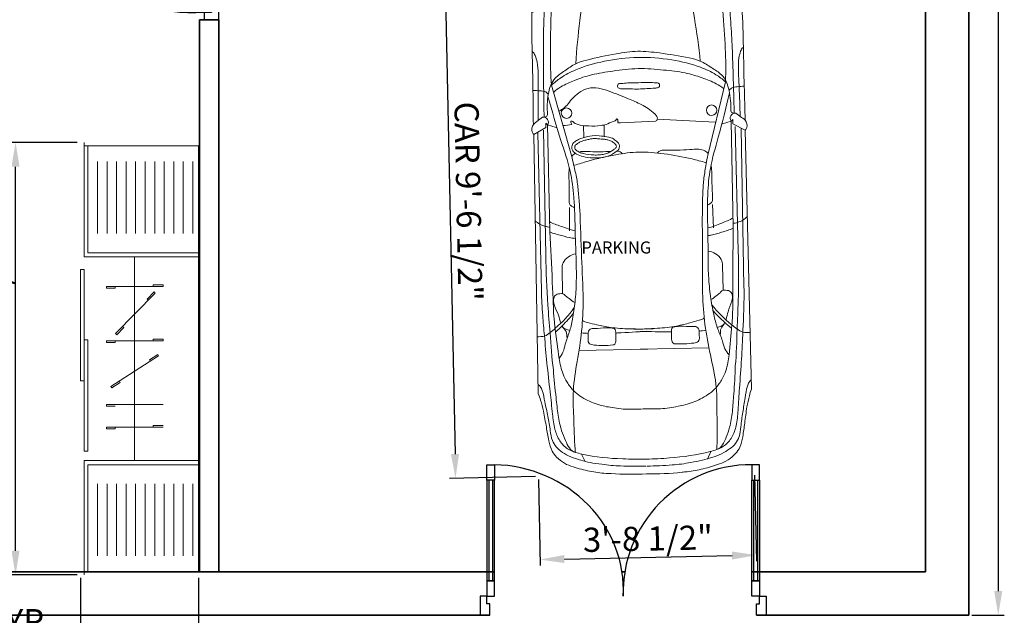
# Model space of a CAD drawing. Units: inches. Extents: x -24887 to 3061, y 1794 to 4919553.
# Tile 10 of 14: x 2858 to 3061, y 1957 to 2080. Entities that reach past the tile are written whole.
import ezdxf

# ---------------------------------------------------------------- set-up
doc = ezdxf.new("R2010")
doc.units = ezdxf.units.IN
for name, color, linetype, lineweight in [('A-ANNO-DIMS', 2, 'Continuous', 18), ('A-AREA-IDEN', 7, 'Continuous', 18), ('A-FLOR-PRKG', 8, 'Continuous', 13), ('A-FURN', 8, 'Continuous', 18), ('door', 4, 'Continuous', 25), ('wall', 7, 'Continuous', 35)]:
    doc.layers.add(name, color=color, linetype=linetype, lineweight=lineweight)
doc.styles.get("Standard").update_dxf_attribs({"font": 'arial.ttf'})
doc.dimstyles.new('ISO-25', dxfattribs={"dimtxt": 5, "dimasz": 5, "dimexe": 1.25, "dimexo": 0.625, "dimtad": 1, "dimdec": 1, "dimlunit": 3, "dimtxsty": 'Standard', "dimcen": 2.5, "dimadec": 0, "dimazin": 0, "dimtfac": 1, "dimtdec": 1, "dimtmove": 0, "dimatfit": 3, "dimfxl": 1, "dimarcsym": 0})

# ---------------------------------------------------------------- blocks, each defined once
blk = doc.blocks.new('A$C34930FF8')
at = {"ltscale": 0.05}
for p, q in [((0, 2252.4), (0, 16.8)), ((600, 2252.4), (0, 2252.4)), ((185.4, 1513), (185.4, 1521.5)), ((237.7, 1513), (237.7, 1521.5)), ((436.7, 1513), (436.7, 1504.4)), ((482.5, 1513), (482.5, 1504.4)), ((227.1, 1479.2), (233.2, 1485.2)), ((263.6, 1441.7), (269.7, 1447.7)), ((398.2, 1303.6), (392.1, 1297.6)), ((434.8, 1266.1), (428.7, 1260.1)), ((185.4, 1229.1), (185.4, 1237.7)), ((237.7, 1229.1), (237.7, 1237.7)), ((436.7, 1228.2), (436.7, 1219.7)), ((482.5, 1228.2), (482.5, 1219.7)), ((209.5, 1150.1), (214.1, 1157.3)), ((253.5, 1121.8), (258.1, 1129)), ((415.3, 1017.6), (410.6, 1010.5)), ((459.3, 989.3), (454.7, 982.1)), ((482.5, 894.9), (482.5, 886.3)), ((237.7, 775.3), (237.7, 783.9)), ((436.7, 775.3), (436.7, 766.8)), ((482.5, 775.3), (482.5, 766.8)), ((600, 16.8), (0, 16.8))]:
    blk.add_line(p, q, dxfattribs=at)
for p, q in [((580, 1690.9), (580, 2252.4)), ((600, 1669.3), (600, 2269.3)), ((30, 1790.9), (30, 2169.3)), ((80, 1790.9), (80, 2169.3)), ((130, 1790.9), (130, 2169.3)), ((180, 1790.9), (180, 2169.3)), ((230, 1790.9), (230, 2169.3)), ((280, 1790.9), (280, 2169.3)), ((330, 1790.9), (330, 2169.3)), ((380, 1790.9), (380, 2169.3)), ((430, 1790.9), (430, 2169.3)), ((480, 1790.9), (480, 2169.3)), ((530, 1790.9), (530, 2169.3)), ((580, 1690.9), (0, 1690.9)), ((600, 1669.3), (0, 1669.3)), ((335.4, 1666.1), (335.4, 603.1)), ((600, 1603.3), (620, 1603.3)), ((600, 1018.7), (600, 1603.3)), ((620, 1603.3), (620, 1018.7)), ((237.7, 1521.5), (185.4, 1521.5)), ((482.5, 1513), (185.4, 1513)), ((436.7, 1504.4), (482.5, 1504.4)), ((434.8, 1266.1), (227.4, 1478.9)), ((269.7, 1447.7), (233.2, 1485.2)), ((428.7, 1260.1), (392.1, 1297.6)), ((237.7, 1237.7), (185.4, 1237.7)), ((482.5, 1228.2), (185.4, 1228.2)), ((436.7, 1219.7), (482.5, 1219.7)), ((600, 1233.4), (580, 1233.4)), ((580, 1233.4), (580, 648.7)), ((600, 648.7), (600, 1233.4)), ((459.3, 989.3), (209.5, 1150.1)), ((258.1, 1129), (214.1, 1157.3)), ((454.7, 982.1), (410.6, 1010.5)), ((620, 1018.7), (600, 1018.7)), ((482.5, 894.9), (185.4, 894.9)), ((436.7, 886.3), (482.5, 886.3)), ((237.7, 783.9), (185.4, 783.9)), ((482.5, 775.3), (185.4, 775.3)), ((436.7, 766.8), (482.5, 766.8)), ((580, 648.7), (600, 648.7)), ((600, 600), (0, 600)), ((580, 578.3), (0, 578.3)), ((580, 578.3), (580, 16.8)), ((600, 600), (600, 0)), ((30, 478.3), (30, 100)), ((80, 478.3), (80, 100)), ((130, 478.3), (130, 100)), ((180, 478.3), (180, 100)), ((230, 478.3), (230, 100)), ((280, 478.3), (280, 100)), ((330, 478.3), (330, 100)), ((380, 478.3), (380, 100)), ((430, 478.3), (430, 100)), ((480, 478.3), (480, 100)), ((530, 478.3), (530, 100))]:
    blk.add_line(p, q)
blk = doc.blocks.new('A$C242571DA')
for p, q in [((1659.9, 1632), (1714.3, 1732.5)), ((1699.9, 1699.4), (2984.7, 1695.8)), ((1714.3, 1732.5), (3817.1, 1739.9)), ((1638.3, 1618.5), (1625.1, 1632)), ((1625.1, 1632), (1659.9, 1632)), ((1638.3, 1618.5), (2503.3, 1618.5)), ((1659.9, 1548.1), (1638.3, 1618.5)), ((1681.8, 1651.6), (2695.2, 1655.3)), ((2503.3, 1618.5), (2861.6, 1607.5)), ((1317.4, 1579.7), (1909.8, 1424.9)), ((3007.2, 1526.5), (2808.1, 1525.2)), ((1644, 1489.1), (1610.4, 1020.2)), ((2311.9, 1454.3), (2500.6, 1456.9)), ((3474.6, 1401.1), (3474.6, 843)), ((4315.2, 1398), (4377.3, 1370.5)), ((1626.1, 1006.5), (1632.8, 719.7)), ((3474.6, 345.6), (3474.6, 903.8)), ((1740.2, 584.9), (1649.3, 586.9)), ((1746.1, 420.6), (1649.3, 420.6)), ((1317.4, 167), (1909.8, 321.9)), ((4315.2, 348.7), (4377.3, 376.3)), ((2311.9, 292.5), (2500.6, 289.8)), ((1659.9, 198.7), (1638.3, 128.2)), ((3007.2, 220.3), (2808.1, 221.6)), ((1638.3, 128.2), (1625.1, 114.7)), ((1625.1, 114.7), (1659.9, 114.7)), ((1638.3, 128.2), (2503.3, 128.2)), ((1659.9, 114.7), (1714.3, 14.2)), ((1681.8, 95.1), (2695.2, 91.4)), ((2503.3, 128.2), (2861.6, 139.2)), ((1699.9, 47.3), (2984.7, 51)), ((1714.3, 14.2), (3817.1, 6.9))]:
    blk.add_line(p, q)
for centre in [(1546.4, 1462.5), (1546.4, 284.2)]:
    blk.add_ellipse(centre, major_axis=(0, 42.9), ratio=0.983266, start_param=4.712389, end_param=10.995574)
for points, knots in [([(0, 873.4), (0, 927.8), (15.6, 1088.6), (25.5, 1309.8), (120.7, 1476.4), (189.2, 1569), (273.5, 1623.1), (369.9, 1666.3), (483, 1694.7), (561.3, 1714.9), (604.6, 1715.7)], [0, 0, 0, 0, 0.16039, 0.479033, 0.632967, 0.722015, 0.817474, 0.927562, 1.03733, 1.167094, 1.167094, 1.167094, 1.167094]), ([(604.6, 1715.7), (545.5, 1714.5), (448.5, 1664.6), (320.8, 1610.6), (225.4, 1521.2), (147.3, 1390.5), (121.7, 1275.2), (113.6, 1208.7)], [0, 0, 0, 0, 0.1772572, 0.3124951, 0.4151678, 0.5597243, 0.7575412, 0.7575412, 0.7575412, 0.7575412]), ([(722.7, 1726.6), (720.8, 1714.9), (694.5, 1689.9), (643, 1671.8), (573.6, 1655.4), (508.5, 1647), (455.2, 1634.7), (428.7, 1627.3), (416.9, 1624.1)], [0, 0, 0, 0, 0.034703, 0.0959761, 0.1659336, 0.2471559, 0.2929944, 0.3295918, 0.3295918, 0.3295918, 0.3295918]), ([(604.6, 1715.7), (642.1, 1723.4), (788.5, 1729.2), (1039.3, 1732.2), (1344.5, 1729.9), (1542, 1733.1), (1633.8, 1733.7)], [0, 0, 0, 0, 0.114897, 0.437061, 0.754269, 1.029686, 1.029686, 1.029686, 1.029686]), ([(1043.6, 1729.2), (1048.6, 1717.9), (1080.9, 1704.2), (1138.6, 1687.6), (1237.7, 1685.6), (1394.7, 1691.3), (1521.7, 1692.4), (1601.5, 1692.7)], [0, 0, 0, 0, 0.0364992, 0.0923739, 0.1867837, 0.3273982, 0.5667068, 0.5667068, 0.5667068, 0.5667068]), ([(1356.8, 1732.2), (1357.1, 1712.8), (1360, 1678.8), (1363.9, 1630.5), (1383.3, 1613.5), (1391, 1607.2)], [0, 0, 0, 0, 1.462159, 2.651105, 3.386321, 3.386321, 3.386321, 3.386321]), ([(1714.3, 1732.5), (1707.7, 1737.6), (1683.3, 1753), (1628.7, 1741.2), (1605.6, 1691.5), (1561.7, 1652.4), (1594.1, 1610.3), (1627.9, 1608.3), (1638.3, 1618.5)], [0, 0, 0, 0, 0.024864, 0.0846267, 0.1362471, 0.1900683, 0.2245199, 0.2681841, 0.2681841, 0.2681841, 0.2681841]), ([(2414.7, 1735), (2424.9, 1723.3), (2447.2, 1698.8), (2461.2, 1657.6), (2468.1, 1629), (2468, 1616.1)], [1.808086, 1.808086, 1.808086, 1.808086, 2.918874, 4.131288, 5.10151, 5.10151, 5.10151, 5.10151]), ([(2984.7, 1695.8), (3051, 1695.6), (3172.1, 1691.3), (3367.4, 1677.6), (3575.2, 1664.3), (3788.2, 1643.6), (3968, 1628.1), (4103.8, 1616.8), (4203.6, 1578.1), (4271.8, 1519.5), (4300.6, 1452.1), (4341.7, 1305.3), (4361.8, 1111.2), (4367.5, 936.8), (4367.5, 873.4)], [0, 0, 0, 0, 0.198873, 0.363323, 0.587433, 0.823543, 1.004622, 1.129816, 1.230113, 1.320655, 1.388577, 1.443334, 1.771447, 1.958652, 1.958652, 1.958652, 1.958652]), ([(3356.5, 1739.4), (3354.9, 1719.2), (3360.8, 1678.2), (3324, 1631.5), (3255.4, 1544.3), (3187.1, 1476.2), (3125.2, 1432.2)], [0, 0, 0, 0, 0.0597371, 0.1139981, 0.1672498, 0.3938869, 0.3938869, 0.3938869, 0.3938869]), ([(3745.3, 1736.8), (3748.5, 1730.1), (3764.2, 1717.1), (3811.5, 1698.6), (3894.7, 1686.7), (4002.9, 1663.2), (4107.9, 1648.7), (4195.8, 1638.3), (4258.6, 1603.2), (4302.1, 1549.7), (4339.9, 1483.8), (4365.2, 1407.6), (4389.6, 1324.4), (4397.9, 1266.9), (4401.8, 1235.2)], [0, 0, 0, 0, 0.0219205, 0.0572122, 0.1522539, 0.2718866, 0.3894011, 0.4710097, 0.5346344, 0.5986698, 0.6733118, 0.758696, 0.8351341, 0.9293726, 0.9293726, 0.9293726, 0.9293726]), ([(3817.1, 1739.9), (3833.2, 1729.7), (3882.9, 1718.2), (3973.3, 1695.2), (4085.1, 1680.5), (4193.8, 1662.8), (4280.6, 1644.3), (4343.9, 1598.1), (4390, 1540.3), (4427.4, 1448.7), (4457.8, 1336.6), (4475.7, 1233.4), (4478.4, 1175.1), (4479.3, 1161.6)], [0, 0, 0, 0, 0.056668, 0.14946, 0.28161, 0.392935, 0.481686, 0.542967, 0.622845, 0.69797, 0.833643, 0.965665, 1.00577, 1.00577, 1.00577, 1.00577]), ([(310.7, 1637.3), (282.5, 1613.7), (230.1, 1569.9), (148.7, 1486.2), (84.8, 1361.3), (60, 1219), (32.6, 1054.3), (25.1, 944.9), (25.1, 873.4)], [0, 0, 0, 0, 0.1095129, 0.2035347, 0.3452507, 0.5161382, 0.6275464, 0.8383798, 0.8383798, 0.8383798, 0.8383798]), ([(426.8, 1656.7), (428.5, 1646.6), (426.9, 1625), (399.8, 1616.6), (368.1, 1593.9), (328, 1564.6), (271.6, 1523.9), (237, 1451.9), (196.2, 1376.7), (183.8, 1314.9), (170, 1279.6), (157.2, 1254.2), (133.3, 1244.4), (118.6, 1242.9)], [0, 0, 0, 0, 0.0304541, 0.0502818, 0.0786089, 0.1479133, 0.1986294, 0.2831705, 0.3780326, 0.4523267, 0.4667809, 0.4902599, 0.5347198, 0.5347198, 0.5347198, 0.5347198]), ([(323.7, 1557.5), (344.8, 1571.9), (400.4, 1585.1), (516, 1606.8), (680.3, 1625.8), (885.4, 1635.7), (1116.8, 1642.2), (1346.1, 1644.2), (1504.7, 1644.7), (1574, 1645.7)], [0, 0, 0, 0, 0.076148, 0.165903, 0.355672, 0.569871, 0.782325, 1.050047, 1.257936, 1.257936, 1.257936, 1.257936]), ([(1555.2, 1617.8), (1527.7, 1617.8), (1472.5, 1620.4), (1392.7, 1608.8), (1318.5, 1591), (1249.4, 1545.5), (1201.4, 1466.7), (1142.8, 1385.7), (1104.8, 1240.4), (1076, 1072.3), (1056.4, 932.4), (1056.4, 873.4)], [0, 0, 0, 0, 0.082256, 0.165174, 0.241383, 0.30939, 0.405348, 0.511507, 0.603349, 0.843635, 1.017671, 1.017671, 1.017671, 1.017671]), ([(3535.9, 1563.1), (3520.1, 1550.9), (3484.4, 1526.1), (3408.2, 1510.9), (3323.4, 1473.1), (3207.9, 1445), (3072.6, 1422.2), (2866.9, 1404.6), (2626.4, 1412.9), (2396.7, 1410.8), (2200.9, 1416.9), (2001.3, 1438.2), (1732.1, 1525.9), (1527.9, 1578.9), (1407.5, 1610.7)], [0, 0, 0, 0, 0.05975, 0.126928, 0.230034, 0.336675, 0.482225, 0.641324, 0.954906, 1.203173, 1.330375, 1.542773, 1.802261, 2.175545, 2.175545, 2.175545, 2.175545]), ([(1574, 1645.7), (1572.9, 1638), (1574.1, 1622), (1559.9, 1618.7), (1555.2, 1617.8)], [0, 0, 0, 0, 0.02274132, 0.03717479, 0.03717479, 0.03717479, 0.03717479]), ([(2424, 1618.7), (2441.5, 1589.9), (2464.2, 1518.9), (2495.4, 1450.9), (2501.6, 1411.3)], [0, 0, 0, 0, 0.1000351, 0.2184418, 0.2184418, 0.2184418, 0.2184418]), ([(2507.7, 1618.4), (2521, 1587.7), (2536.6, 1527.1), (2559.6, 1458.5), (2563.3, 1420.6), (2563.8, 1411.4)], [0, 0, 0, 0, 2.528586, 4.711885, 5.408215, 5.408215, 5.408215, 5.408215]), ([(2695.2, 1655.3), (2829.9, 1655.3), (3041.2, 1651.4), (3351.3, 1630.7), (3527.5, 1623.2), (3626.6, 1612)], [0, 0, 0, 0, 0.4042759, 0.6333827, 0.9326252, 0.9326252, 0.9326252, 0.9326252]), ([(2861.6, 1607.5), (2921.1, 1607.3), (3047.2, 1600.8), (3191.4, 1602), (3356.6, 1584.1), (3498.3, 1570.6), (3623.2, 1549.4), (3664.1, 1533.3)], [0, 0, 0, 0, 0.1783018, 0.3787173, 0.431954, 0.6762374, 0.8077184, 0.8077184, 0.8077184, 0.8077184]), ([(3248.1, 1545.2), (3226.9, 1550.4), (3176.1, 1562.1), (3113.7, 1592.9), (3052.6, 1605.3), (3010.4, 1578.8), (3010.3, 1545.3), (3010.3, 1515.9), (3033.7, 1500.1), (3052.6, 1465.2), (3078.9, 1443.5), (3084, 1424.4)], [0, 0, 0, 0, 0.0655106, 0.1550445, 0.2094604, 0.2438604, 0.287164, 0.3001388, 0.3275984, 0.3616951, 0.4200969, 0.4200969, 0.4200969, 0.4200969]), ([(3626.6, 1612), (3702.5, 1609.1), (3826.2, 1596.8), (3991.4, 1583.2), (4111.7, 1562.4), (4212.2, 1522.7), (4290.4, 1488), (4300.7, 1447.5)], [0, 0, 0, 0, 0.2277977, 0.3719478, 0.4996814, 0.5863441, 0.709615, 0.709615, 0.709615, 0.709615]), ([(1317.4, 1579.7), (1227.8, 1586.1), (1036, 1584.8), (741.2, 1572.5), (486.1, 1553.3), (333.3, 1534.3), (283.3, 1528.5)], [0, 0, 0, 0, 0.269375, 0.574535, 0.885339, 1.036319, 1.036319, 1.036319, 1.036319]), ([(1317.4, 1579.7), (1296.6, 1555.5), (1247.9, 1494.4), (1177.6, 1350.5), (1124.2, 1137.4), (1105.5, 964.9), (1105.5, 873.4)], [0, 0, 0, 0, 0.0947759, 0.2311242, 0.4700259, 0.7400315, 0.7400315, 0.7400315, 0.7400315]), ([(1372.8, 1563.1), (1357.2, 1545), (1321.6, 1490.1), (1277, 1385.7), (1232.8, 1244.2), (1211.1, 1069.4), (1196.8, 942.4), (1196.8, 873.4)], [0, 0, 0, 0, 0.0708922, 0.1925846, 0.3348457, 0.5072814, 0.7109928, 0.7109928, 0.7109928, 0.7109928]), ([(2808.1, 1525.2), (2791.9, 1525.1), (2751.9, 1519.7), (2710.6, 1472.6), (2690, 1431.1), (2690.5, 1409.6)], [0, 0, 0, 0, 0.0486628, 0.1144515, 0.1777721, 0.1777721, 0.1777721, 0.1777721]), ([(3319, 1587.1), (3303.3, 1568.1), (3256.9, 1516.7), (3206.7, 1467.3), (3171.4, 1439.5)], [0, 0, 0, 0, 1.868162, 5.271297, 5.271297, 5.271297, 5.271297]), ([(3275.5, 1532.8), (3287.5, 1528.3), (3299.8, 1504.9), (3308.4, 1482.5), (3311.7, 1472.6)], [0, 0, 0, 0, 0.983949, 1.771691, 1.771691, 1.771691, 1.771691]), ([(3372.2, 1495.3), (3354.4, 1496.8), (3316, 1494.7), (3291.6, 1525.8), (3275.5, 1532.8)], [0, 0, 0, 0, 0.0535488, 0.1060573, 0.1060573, 0.1060573, 0.1060573]), ([(3664.1, 1533.3), (3687, 1526), (3734.8, 1502.3), (3816.7, 1444.8), (3884.1, 1342.9), (3925.1, 1239.9), (3937.3, 1177), (3940.4, 1157.6)], [0, 0, 0, 0, 0.0720749, 0.1581284, 0.2958089, 0.4262456, 0.4842292, 0.4842292, 0.4842292, 0.4842292]), ([(1909.8, 1424.9), (1933.5, 1418.7), (1995.6, 1407.6), (2094.4, 1385.8), (2211.8, 1377.1), (2419, 1366.9), (2704.7, 1366.5), (3032.7, 1354.2), (3316.2, 1371), (3558.7, 1415.9), (3789.1, 1461.7), (4028.9, 1452.9), (4196.2, 1455.2), (4292.7, 1447.9), (4300.7, 1447.5)], [0, 0, 0, 0, 0.073325, 0.188896, 0.303039, 0.425821, 0.811242, 1.159737, 1.41058, 1.660623, 1.899627, 2.11145, 2.377727, 2.401703, 2.401703, 2.401703, 2.401703]), ([(1997.2, 1450.5), (2039.7, 1454.5), (2126.7, 1451.9), (2219.8, 1454.5), (2287.1, 1456.9), (2305.7, 1434.4), (2313.2, 1419.9), (2315.8, 1413.5)], [0, 0, 0, 0, 3.267856, 6.568708, 7.399663, 8.099385, 8.621705, 8.621705, 8.621705, 8.621705]), ([(113.6, 1208.7), (215.2, 1238.6), (443.2, 1284.9), (788, 1338.7), (1029.5, 1370.7), (1146.4, 1378.6)], [0, 0, 0, 0, 0.317374, 0.69576, 1.04714, 1.04714, 1.04714, 1.04714]), ([(1898.5, 1426.2), (1889, 1420.6), (1871, 1397.2), (1856.4, 1345.2), (1867.7, 1233.5), (1864.3, 1132.3), (1863, 1038.5), (1876.9, 1022.3), (1884.5, 1015.7)], [0, 0, 0, 0, 0.842998, 2.122875, 3.997599, 9.174838, 10.012722, 10.751336, 10.751336, 10.751336, 10.751336]), ([(1969.6, 1407.3), (1960.5, 1369.8), (1927, 1259.1), (1890.9, 1078.4), (1874.3, 933), (1874.3, 864.4)], [0, 0, 0, 0, 0.1139079, 0.3411539, 0.543502, 0.543502, 0.543502, 0.543502]), ([(3231.5, 1368.3), (3240.8, 1356.2), (3253.1, 1315.7), (3271.9, 1240.7), (3297.9, 1127.9), (3310.5, 974.6), (3311.2, 858.3), (3311.6, 794.4)], [0, 0, 0, 0, 0.0451009, 0.1211996, 0.2308505, 0.385263, 0.5739042, 0.5739042, 0.5739042, 0.5739042]), ([(3294.8, 1174.5), (3294.8, 1207.4), (3299.6, 1249.5), (3298.3, 1303.9), (3326.3, 1329), (3363.9, 1320.7), (3399.3, 1329.3), (3422.1, 1315.7), (3430.7, 1297.9), (3438.7, 1234.2), (3439.6, 1174.4), (3434.7, 1112.2), (3418.9, 1102), (3395.9, 1098.6), (3362.6, 1100.9), (3331.1, 1096.6), (3298.8, 1107.6), (3297.3, 1140.3), (3294.8, 1160.9), (3294.8, 1174.5)], [0, 0, 0, 0, 0.0969044, 0.1295913, 0.1506192, 0.1985921, 0.2360698, 0.2557908, 0.2719711, 0.2929882, 0.44406, 0.4519132, 0.4720918, 0.4918599, 0.5228758, 0.5707096, 0.5892096, 0.6145759, 0.654681, 0.654681, 0.654681, 0.654681]), ([(113.6, 1208.7), (103.3, 1207), (83.6, 1187.6), (76.5, 1122.2), (68.2, 1017.3), (53.4, 925), (53.4, 873.4)], [0, 0, 0, 0, 0.0314754, 0.0702057, 0.1915753, 0.3439346, 0.3439346, 0.3439346, 0.3439346]), ([(135.5, 1213.1), (139.1, 1211.8), (138.4, 1193.3), (132.6, 1168.3), (118.8, 1111.9), (115.6, 1058.9), (109, 974.6), (102.4, 920.1), (102.4, 873.4)], [0, 0, 0, 0, 0.0114788, 0.0403472, 0.0875838, 0.1755608, 0.1991501, 0.3369659, 0.3369659, 0.3369659, 0.3369659]), ([(4401.8, 1235.2), (4411.9, 1185.3), (4421.6, 1065.8), (4424.1, 946.5), (4424.1, 878)], [0, 0, 0, 0, 0.1502861, 0.3522699, 0.3522699, 0.3522699, 0.3522699]), ([(3940.4, 1157.6), (3949.9, 1111), (3964.3, 1016.4), (3960.5, 921), (3959.8, 873.4)], [0, 0, 0, 0, 0.140379, 0.2808468, 0.2808468, 0.2808468, 0.2808468]), ([(1311.3, 873.4), (1311.2, 902.4), (1309.2, 950.9), (1315, 1002.2), (1314.2, 1039.4), (1332.1, 1044.9), (1345.7, 1044.2), (1356.8, 1028.5), (1359.2, 970.2), (1361.5, 917.6), (1362.9, 873.4)], [0, 0, 0, 0, 0.0857277, 0.1381048, 0.1641986, 0.1769751, 0.1890325, 0.2028129, 0.2286049, 0.3592554, 0.3592554, 0.3592554, 0.3592554]), ([(3339.2, 1099), (3339.1, 1094.8), (3336.4, 1010.6), (3333.2, 926.3), (3330, 846.2)], [11.235438, 11.235438, 11.235438, 11.235438, 11.552536, 17.586883, 17.586883, 17.586883, 17.586883]), ([(1626.1, 1006.5), (1623.5, 1013), (1603.1, 1029.4), (1559.1, 995), (1523, 951.9), (1480.3, 878.3), (1430.5, 774.3), (1385.5, 658.5), (1343.7, 551.3), (1343, 461.7), (1380.3, 386.9), (1428.2, 329.9), (1480.1, 294.6), (1509.8, 257.4), (1524.8, 232.6), (1528, 222.1)], [0, 0, 0, 0, 0.527288, 1.647451, 3.487558, 5.099073, 7.968657, 12.238313, 14.475187, 16.613757, 18.744202, 20.639343, 22.223389, 23.452731, 24.286529, 24.286529, 24.286529, 24.286529]), ([(3231.5, 378.5), (3240.8, 390.5), (3253.1, 431), (3271.9, 506.1), (3297.9, 618.9), (3310.5, 772.1), (3311.2, 888.4), (3311.6, 952.4)], [0, 0, 0, 0, 0.0451009, 0.1211996, 0.2308505, 0.385263, 0.5739042, 0.5739042, 0.5739042, 0.5739042]), ([(3339.2, 647.8), (3339.1, 652), (3336.4, 736.2), (3333.2, 820.5), (3330, 900.6)], [11.235438, 11.235438, 11.235438, 11.235438, 11.552536, 17.586883, 17.586883, 17.586883, 17.586883]), ([(0, 873.4), (0, 819), (15.6, 658.1), (25.5, 437), (120.7, 270.3), (189.2, 177.8), (273.5, 123.7), (369.9, 80.4), (483, 52), (561.3, 31.9), (604.6, 31)], [0, 0, 0, 0, 0.16039, 0.479033, 0.632967, 0.722015, 0.817474, 0.927562, 1.03733, 1.167094, 1.167094, 1.167094, 1.167094]), ([(310.7, 109.5), (282.5, 133.1), (230.1, 176.9), (148.7, 260.5), (84.8, 385.5), (60, 527.8), (32.6, 692.4), (25.1, 801.9), (25.1, 873.4)], [0, 0, 0, 0, 0.1095129, 0.2035347, 0.3452507, 0.5161382, 0.6275464, 0.8383798, 0.8383798, 0.8383798, 0.8383798]), ([(113.6, 538.1), (103.3, 539.8), (83.6, 559.2), (76.5, 624.5), (68.2, 729.4), (53.4, 821.7), (53.4, 873.4)], [0, 0, 0, 0, 0.0314754, 0.0702057, 0.1915753, 0.3439346, 0.3439346, 0.3439346, 0.3439346]), ([(135.5, 533.6), (139.1, 534.9), (138.4, 553.4), (132.6, 578.4), (118.8, 634.9), (115.6, 687.8), (109, 772.2), (102.4, 826.7), (102.4, 873.4)], [0, 0, 0, 0, 0.0114788, 0.0403472, 0.0875838, 0.1755608, 0.1991501, 0.3369659, 0.3369659, 0.3369659, 0.3369659]), ([(1555.2, 129), (1527.7, 129), (1472.5, 126.3), (1392.7, 138), (1318.5, 155.7), (1249.4, 201.3), (1201.4, 280.1), (1142.8, 361.1), (1104.8, 506.4), (1076, 674.5), (1056.4, 814.4), (1056.4, 873.4)], [0, 0, 0, 0, 0.082256, 0.165174, 0.241383, 0.30939, 0.405348, 0.511507, 0.603349, 0.843635, 1.017671, 1.017671, 1.017671, 1.017671]), ([(1317.4, 167), (1296.6, 191.2), (1247.9, 252.4), (1177.6, 396.3), (1124.2, 609.4), (1105.5, 781.8), (1105.5, 873.4)], [0, 0, 0, 0, 0.0947759, 0.2311242, 0.4700259, 0.7400315, 0.7400315, 0.7400315, 0.7400315]), ([(1372.8, 183.6), (1357.2, 201.8), (1321.6, 256.7), (1277, 361), (1232.8, 502.6), (1211.1, 677.3), (1196.8, 804.3), (1196.8, 873.4)], [0, 0, 0, 0, 0.0708922, 0.1925846, 0.3348457, 0.5072814, 0.7109928, 0.7109928, 0.7109928, 0.7109928]), ([(1311.3, 873.4), (1311.2, 844.3), (1309.2, 795.8), (1315, 744.6), (1314.2, 707.4), (1332.1, 701.9), (1345.7, 702.6), (1356.8, 718.2), (1359.2, 776.6), (1361.5, 829.1), (1362.9, 873.4)], [0, 0, 0, 0, 0.0857277, 0.1381048, 0.1641986, 0.1769751, 0.1890325, 0.2028129, 0.2286049, 0.3592554, 0.3592554, 0.3592554, 0.3592554]), ([(1969.6, 339.5), (1960.5, 377), (1926.9, 487.6), (1892.9, 662.7), (1874.3, 801.8), (1874.3, 864.4)], [0, 0, 0, 0, 0.1139079, 0.3411539, 0.5260188, 0.5260188, 0.5260188, 0.5260188]), ([(2984.7, 51), (3051, 51.1), (3172.1, 55.5), (3367.4, 69.2), (3575.2, 82.5), (3788.2, 103.1), (3968, 118.7), (4103.8, 130), (4203.6, 168.6), (4271.8, 227.3), (4300.6, 294.7), (4341.7, 441.5), (4361.8, 635.5), (4367.5, 809.9), (4367.5, 873.4)], [0, 0, 0, 0, 0.198873, 0.363323, 0.587433, 0.823543, 1.004622, 1.129816, 1.230113, 1.320655, 1.388577, 1.443334, 1.771447, 1.958652, 1.958652, 1.958652, 1.958652]), ([(3940.4, 589.1), (3949.9, 635.7), (3964.3, 730.4), (3960.5, 825.8), (3959.8, 873.4)], [0, 0, 0, 0, 0.140379, 0.2808468, 0.2808468, 0.2808468, 0.2808468]), ([(4401.8, 511.5), (4411.9, 561.5), (4421.6, 681), (4424.1, 800.3), (4424.1, 868.8)], [0, 0, 0, 0, 0.1502861, 0.3522699, 0.3522699, 0.3522699, 0.3522699]), ([(1639.2, 326.1), (1635.3, 323.6), (1629, 318.4), (1613.1, 314.9), (1612, 324.2), (1613.2, 330.4), (1619, 337.5), (1629, 345.7), (1637.9, 366.1), (1649, 404.8), (1656.3, 472.9), (1656.2, 543.1), (1644.6, 610.9), (1623, 651.2), (1615, 684.3), (1598.5, 691.2), (1604, 696.6), (1610.3, 699.7), (1618.8, 698.9), (1625.9, 701.3), (1638.1, 698.6), (1633, 713.4), (1632.8, 719.7)], [0, 0, 0, 0, 0.0138597, 0.0278304, 0.0329137, 0.0379971, 0.0465756, 0.0592704, 0.0762214, 0.1105991, 0.1789801, 0.2766959, 0.3173629, 0.3800771, 0.4110544, 0.4160421, 0.4210284, 0.4277212, 0.4387433, 0.4448131, 0.4508005, 0.4694463, 0.4694463, 0.4694463, 0.4694463]), ([(1863.4, 685.6), (1863.6, 693.5), (1865.3, 711), (1876.9, 724.5), (1884.5, 731)], [9.436432, 9.436432, 9.436432, 9.436432, 10.012722, 10.751336, 10.751336, 10.751336, 10.751336]), ([(1740.2, 584.9), (1737.8, 571.7), (1749.5, 644.3), (1766.4, 664.5), (1792.2, 700.2), (1821.5, 709.7), (1853.1, 703.9), (1874, 668.4), (1904.5, 622.6), (1915.6, 557.2), (1915.1, 484.2), (1905.7, 417.6), (1884.9, 362.8), (1859.3, 329.1), (1831.3, 318.1), (1810.8, 322.7), (1792.2, 329.3), (1777.9, 350.3), (1753, 385.9), (1737.9, 465.8), (1728.8, 497.3), (1742.4, 597.6), (1740.2, 584.9)], [0, 0, 0, 0, 0.03969, 0.089634, 0.13125, 0.1542862, 0.1797268, 0.2207266, 0.2680991, 0.3447665, 0.4095645, 0.4843001, 0.541515, 0.5817687, 0.6060665, 0.6262474, 0.6436722, 0.6634686, 0.6988791, 0.7758465, 0.8696394, 0.907731, 0.907731, 0.907731, 0.907731]), ([(1764.9, 587), (1765.6, 590.8), (1766.4, 595.5), (1768.5, 605.7), (1769.7, 611.3), (1773.4, 626.6), (1775.6, 633), (1779.7, 642.1), (1781.6, 644.9), (1785.7, 650.6), (1787.1, 652.5), (1793, 660.3), (1797.4, 666.2), (1804.2, 673.7), (1806.8, 676.1), (1811.1, 679.4), (1812.9, 680.5), (1816.8, 682.1), (1818.8, 682.7), (1824.4, 683.5), (1828.3, 683.2), (1832.5, 682), (1833.6, 681.5), (1836, 680.2), (1837.9, 678.7), (1842.4, 673.7), (1844.9, 670.1), (1850.3, 661.7), (1853.4, 656.6), (1859.3, 647.3), (1862.1, 642.8), (1868.3, 632.6), (1871.4, 626.9), (1876.7, 615.7), (1878.9, 609.8), (1882.8, 597.4), (1884.4, 590.8), (1888.3, 570.5), (1889.7, 556.1), (1891.2, 527.4), (1891.1, 513.1), (1888.9, 470), (1885.1, 441.2), (1874.3, 404), (1870.6, 393.8), (1863.5, 378.7), (1860.6, 373.4), (1854.4, 363.6), (1851.2, 359.2), (1845, 352.6), (1842, 350.2), (1835.8, 346.4), (1832.6, 345.3), (1828.8, 344.6), (1827.9, 344.6), (1824.6, 344.9), (1822.6, 345.2), (1817.8, 346.4), (1814.9, 347.3), (1810.9, 348.7), (1809.4, 349.4), (1808.3, 350.1), (1808.1, 350.2), (1807.3, 351), (1806.7, 351.6), (1804.7, 354), (1803.1, 356.2), (1799.6, 361.3), (1798, 363.7), (1794.9, 368.2), (1793.4, 370.4), (1789.2, 376.9), (1786.7, 381), (1782.4, 389.3), (1780.5, 393.6), (1776.9, 403), (1775.2, 408), (1770.7, 423.5), (1768.3, 434.2), (1764.9, 450.5), (1763.6, 456.4), (1761.4, 466.8), (1760.4, 471.4), (1758.1, 484.4), (1757.3, 492.6), (1757.5, 510.7), (1757.8, 516.5), (1758.6, 528.4), (1759.1, 534.3), (1761.1, 553.9), (1763.1, 570.6), (1764.4, 581.5), (1764.6, 583), (1764.7, 585), (1764.8, 585.5), (1764.8, 586.5), (1764.8, 586.7), (1764.9, 587)], [0.497033, 0.497033, 0.497033, 0.497033, 0.723444, 0.723444, 0.974636, 0.974636, 1.50964, 1.50964, 2.044645, 2.044645, 2.271061, 2.271061, 2.862376, 2.862376, 3.217654, 3.217654, 3.537253, 3.537253, 3.856852, 3.856852, 4.368613, 4.368613, 4.584627, 4.584627, 4.99269, 4.99269, 5.400753, 5.400753, 5.808816, 5.808816, 6.216879, 6.216879, 6.778716, 6.778716, 7.350371, 7.350371, 7.922025, 7.922025, 9.065335, 9.065335, 10.208644, 10.208644, 12.495263, 12.495263, 13.409896, 13.409896, 13.929088, 13.929088, 14.44828, 14.44828, 14.909885, 14.909885, 15.371489, 15.371489, 15.62524, 15.62524, 15.87899, 15.87899, 16.120875, 16.120875, 16.36276, 16.36276, 16.51635, 16.51635, 16.669941, 16.669941, 16.921521, 16.921521, 17.136676, 17.136676, 17.351831, 17.351831, 17.782142, 17.782142, 18.204974, 18.204974, 18.627807, 18.627807, 19.473473, 19.473473, 19.978923, 19.978923, 20.484372, 20.484372, 21.475119, 21.475119, 21.859144, 21.859144, 22.162884, 22.162884, 22.770362, 22.770362, 22.900493, 22.900493, 22.951221, 22.951221, 22.964298, 22.964298, 22.964298, 22.964298]), ([(3294.8, 572.3), (3294.8, 539.4), (3299.6, 497.2), (3298.3, 442.9), (3326.3, 417.8), (3363.9, 426), (3399.3, 417.5), (3422.1, 431), (3430.7, 448.9), (3438.7, 512.5), (3439.6, 572.4), (3434.7, 634.6), (3418.9, 644.7), (3395.9, 648.2), (3362.6, 645.9), (3331.1, 650.1), (3298.8, 639.2), (3297.3, 606.5), (3294.8, 585.9), (3294.8, 572.3)], [0, 0, 0, 0, 0.0969044, 0.1295913, 0.1506192, 0.1985921, 0.2360698, 0.2557908, 0.2719711, 0.2929882, 0.44406, 0.4519132, 0.4720918, 0.4918599, 0.5228758, 0.5707096, 0.5892096, 0.6145759, 0.654681, 0.654681, 0.654681, 0.654681]), ([(1863.7, 379.4), (1862.6, 384.2), (1857.6, 413.7), (1866.5, 501.6), (1865.2, 581.4), (1864.1, 639.5)], [1.749253, 1.749253, 1.749253, 1.749253, 2.122875, 3.997599, 8.307432, 8.307432, 8.307432, 8.307432]), ([(3664.1, 213.5), (3687, 220.8), (3734.8, 244.4), (3816.7, 302), (3884.1, 403.8), (3925.1, 506.9), (3937.3, 569.7), (3940.4, 589.1)], [0, 0, 0, 0, 0.0720749, 0.1581284, 0.2958089, 0.4262456, 0.4842292, 0.4842292, 0.4842292, 0.4842292]), ([(3817.1, 6.9), (3833.2, 17), (3882.9, 28.6), (3973.3, 51.5), (4085.1, 66.3), (4193.8, 84), (4280.6, 102.4), (4343.9, 148.6), (4390, 206.4), (4427.4, 298), (4457.8, 410.1), (4475.7, 513.3), (4478.4, 571.6), (4479.3, 585.2)], [0, 0, 0, 0, 0.056668, 0.14946, 0.28161, 0.392935, 0.481686, 0.542967, 0.622845, 0.69797, 0.833643, 0.965665, 1.00577, 1.00577, 1.00577, 1.00577]), ([(604.6, 31), (545.5, 32.3), (448.5, 82.2), (320.8, 136.1), (225.4, 225.5), (147.3, 356.2), (121.7, 471.5), (113.6, 538.1)], [0, 0, 0, 0, 0.1772572, 0.3124951, 0.4151678, 0.5597243, 0.7575412, 0.7575412, 0.7575412, 0.7575412]), ([(113.6, 538.1), (215.2, 508.2), (443.2, 461.9), (788, 408.1), (1029.5, 376), (1146.4, 368.2)], [0, 0, 0, 0, 0.317374, 0.69576, 1.04714, 1.04714, 1.04714, 1.04714]), ([(426.8, 90), (428.5, 100.2), (426.9, 121.8), (399.8, 130.1), (368.1, 152.8), (328, 182.2), (271.6, 222.8), (237, 294.9), (196.2, 370.1), (183.8, 431.9), (170, 467.2), (157.2, 492.6), (133.3, 502.4), (118.6, 503.9)], [0, 0, 0, 0, 0.0304541, 0.0502818, 0.0786089, 0.1479133, 0.1986294, 0.2831705, 0.3780326, 0.4523267, 0.4667809, 0.4902599, 0.5347198, 0.5347198, 0.5347198, 0.5347198]), ([(3745.3, 10), (3748.5, 16.7), (3764.2, 29.7), (3811.5, 48.1), (3894.7, 60.1), (4002.9, 83.6), (4107.9, 98), (4195.8, 108.4), (4258.6, 143.5), (4302.1, 197), (4339.9, 262.9), (4365.2, 339.2), (4389.6, 422.4), (4397.9, 479.8), (4401.8, 511.5)], [0, 0, 0, 0, 0.0219205, 0.0572122, 0.1522539, 0.2718866, 0.3894011, 0.4710097, 0.5346344, 0.5986698, 0.6733118, 0.758696, 0.8351341, 0.9293726, 0.9293726, 0.9293726, 0.9293726]), ([(3535.9, 183.7), (3520.1, 195.9), (3484.4, 220.6), (3408.2, 235.8), (3323.4, 273.7), (3207.9, 301.8), (3072.6, 324.6), (2866.9, 342.1), (2626.4, 333.8), (2396.7, 335.9), (2200.9, 329.9), (2001.3, 308.6), (1732.1, 220.8), (1527.9, 167.8), (1407.5, 136)], [0, 0, 0, 0, 0.05975, 0.126928, 0.230034, 0.336675, 0.482225, 0.641324, 0.954906, 1.203173, 1.330375, 1.542773, 1.802261, 2.175545, 2.175545, 2.175545, 2.175545]), ([(1898.5, 320.6), (1889, 326.2), (1880.8, 336.8), (1874.8, 348.3), (1874, 349.7)], [0, 0, 0, 0, 0.8429982, 0.9626806, 0.9626806, 0.9626806, 0.9626806]), ([(1909.8, 321.9), (1933.5, 328.1), (1995.6, 339.2), (2094.4, 361), (2211.8, 369.6), (2419, 379.8), (2704.7, 380.3), (3032.7, 392.6), (3316.2, 375.8), (3558.7, 330.9), (3789.1, 285.1), (4028.9, 293.9), (4196.2, 291.5), (4292.7, 298.8), (4300.7, 299.2)], [0, 0, 0, 0, 0.073325, 0.188896, 0.303039, 0.425821, 0.811242, 1.159737, 1.41058, 1.660623, 1.899627, 2.11145, 2.377727, 2.401703, 2.401703, 2.401703, 2.401703]), ([(1997.2, 296.3), (2039.7, 292.2), (2126.7, 294.9), (2219.8, 292.3), (2287.1, 289.9), (2305.7, 312.3), (2313.2, 326.9), (2315.8, 333.2)], [0, 0, 0, 0, 3.267856, 6.568708, 7.399663, 8.099385, 8.621705, 8.621705, 8.621705, 8.621705]), ([(2424, 128), (2441.5, 156.9), (2464.2, 227.8), (2495.4, 295.8), (2501.6, 335.5)], [0, 0, 0, 0, 0.1000351, 0.2184418, 0.2184418, 0.2184418, 0.2184418]), ([(2507.7, 128.3), (2521, 159.1), (2536.6, 219.7), (2559.6, 288.3), (2563.3, 326.1), (2563.8, 335.3)], [0, 0, 0, 0, 2.528586, 4.711885, 5.408215, 5.408215, 5.408215, 5.408215]), ([(2808.1, 221.6), (2791.9, 221.6), (2751.9, 227.1), (2710.6, 274.2), (2690, 315.7), (2690.5, 337.1)], [0, 0, 0, 0, 0.0486628, 0.1144515, 0.1777721, 0.1777721, 0.1777721, 0.1777721]), ([(3248.1, 201.6), (3226.9, 196.3), (3176.1, 184.7), (3113.7, 153.8), (3052.6, 141.4), (3010.4, 168), (3010.3, 201.5), (3010.3, 230.9), (3033.7, 246.6), (3052.6, 281.6), (3078.9, 303.2), (3084, 322.4)], [0, 0, 0, 0, 0.0655106, 0.1550445, 0.2094604, 0.2438604, 0.287164, 0.3001388, 0.3275984, 0.3616951, 0.4200969, 0.4200969, 0.4200969, 0.4200969]), ([(3356.5, 7.4), (3354.9, 27.5), (3360.8, 68.5), (3324, 115.2), (3255.4, 202.5), (3187.1, 270.5), (3125.2, 314.6)], [0, 0, 0, 0, 0.0597371, 0.1139981, 0.1672498, 0.3938869, 0.3938869, 0.3938869, 0.3938869]), ([(3319, 159.7), (3303.3, 178.6), (3256.9, 230), (3206.7, 279.5), (3171.4, 307.2)], [0, 0, 0, 0, 1.868162, 5.271297, 5.271297, 5.271297, 5.271297]), ([(3275.5, 214), (3287.5, 218.5), (3299.8, 241.9), (3308.4, 264.3), (3311.7, 274.2)], [0, 0, 0, 0, 0.983949, 1.771691, 1.771691, 1.771691, 1.771691]), ([(3372.2, 251.5), (3354.4, 249.9), (3316, 252), (3291.6, 220.9), (3275.5, 214)], [0, 0, 0, 0, 0.0535488, 0.1060573, 0.1060573, 0.1060573, 0.1060573]), ([(3626.6, 134.7), (3702.5, 137.7), (3826.2, 149.9), (3991.4, 163.5), (4111.7, 184.4), (4212.2, 224.1), (4290.4, 258.8), (4300.7, 299.2)], [0, 0, 0, 0, 0.2277977, 0.3719478, 0.4996814, 0.5863441, 0.709615, 0.709615, 0.709615, 0.709615]), ([(1317.4, 167), (1227.8, 160.7), (1036, 161.9), (741.2, 174.2), (486.1, 193.4), (333.3, 212.5), (283.3, 218.3)], [0, 0, 0, 0, 0.269375, 0.574535, 0.885339, 1.036319, 1.036319, 1.036319, 1.036319]), ([(323.7, 189.2), (344.8, 174.9), (400.4, 161.7), (516, 139.9), (680.3, 121), (885.4, 111), (1116.8, 104.5), (1346.1, 102.5), (1504.7, 102), (1574, 101.1)], [0, 0, 0, 0, 0.076148, 0.165903, 0.355672, 0.569871, 0.782325, 1.050047, 1.257936, 1.257936, 1.257936, 1.257936]), ([(2861.6, 139.2), (2921.1, 139.4), (3047.2, 146), (3191.4, 144.8), (3356.6, 162.6), (3498.3, 176.1), (3623.2, 197.4), (3664.1, 213.5)], [0, 0, 0, 0, 0.1783018, 0.3787173, 0.431954, 0.6762374, 0.8077184, 0.8077184, 0.8077184, 0.8077184]), ([(722.7, 20.2), (720.8, 31.8), (694.5, 56.8), (643, 75), (573.6, 91.4), (508.5, 99.8), (455.2, 112.1), (428.7, 119.5), (416.9, 122.6)], [0, 0, 0, 0, 0.034703, 0.0959761, 0.1659336, 0.2471559, 0.2929944, 0.3295918, 0.3295918, 0.3295918, 0.3295918]), ([(1356.8, 14.5), (1357.1, 33.9), (1360, 68), (1363.9, 116.3), (1383.3, 133.2), (1391, 139.5)], [0, 0, 0, 0, 1.462159, 2.651105, 3.386321, 3.386321, 3.386321, 3.386321]), ([(1574, 101.1), (1572.9, 108.7), (1574.1, 124.8), (1559.9, 128), (1555.2, 129)], [0, 0, 0, 0, 0.02274132, 0.03717479, 0.03717479, 0.03717479, 0.03717479]), ([(1714.3, 14.2), (1707.7, 9.2), (1683.3, -6.3), (1628.7, 5.5), (1605.6, 55.3), (1561.7, 94.4), (1594.1, 136.5), (1627.9, 138.5), (1638.3, 128.2)], [0, 0, 0, 0, 0.024864, 0.0846267, 0.1362471, 0.1900683, 0.2245199, 0.2681841, 0.2681841, 0.2681841, 0.2681841]), ([(2414.7, 11.8), (2424.9, 23.5), (2447.2, 48), (2461.2, 89.1), (2468.1, 117.8), (2468, 130.7)], [1.808086, 1.808086, 1.808086, 1.808086, 2.918874, 4.131288, 5.10151, 5.10151, 5.10151, 5.10151]), ([(2695.2, 91.4), (2829.9, 91.5), (3041.2, 95.4), (3351.3, 116.1), (3527.5, 123.5), (3626.6, 134.7)], [0, 0, 0, 0, 0.4042759, 0.6333827, 0.9326252, 0.9326252, 0.9326252, 0.9326252]), ([(604.6, 31), (642.1, 23.4), (788.5, 17.5), (1039.3, 14.6), (1344.5, 16.8), (1542, 13.6), (1633.8, 13.1)], [0, 0, 0, 0, 0.114897, 0.437061, 0.754269, 1.029686, 1.029686, 1.029686, 1.029686]), ([(1043.6, 17.6), (1048.6, 28.9), (1080.9, 42.6), (1138.6, 59.2), (1237.7, 61.2), (1394.7, 55.4), (1521.7, 54.3), (1601.5, 54.1)], [0, 0, 0, 0, 0.0364992, 0.0923739, 0.1867837, 0.3273982, 0.5667068, 0.5667068, 0.5667068, 0.5667068])]:
    blk.add_open_spline(points, degree=3, knots=knots)
for points in [[(283.3, 1528.5), (267.8, 1524.6), (251.4, 1527.5), (235.4, 1528.5)], [(3331.9, 1378.1), (3334.2, 1360.4), (3335.9, 1342.5), (3337.3, 1324.5)], [(4479.3, 1161.6), (4491, 1066.2), (4488, 969.5), (4488, 873.4)], [(4479.3, 585.2), (4491, 680.6), (4488, 777.3), (4488, 873.4)], [(3331.9, 368.6), (3334.2, 386.4), (3335.9, 404.3), (3337.3, 422.2)], [(1646.2, 253.1), (1647.8, 277.5), (1640, 301.6), (1639.2, 326.1)], [(283.3, 218.3), (267.8, 222.1), (251.4, 219.2), (235.4, 218.3)]]:
    blk.add_open_spline(points, degree=3)
blk = doc.blocks.new('*D33')
at = {"layer": 'A-ANNO-DIMS', "color": 0, "lineweight": -2, "transparency": 16777216}
for p, q in [((3054.55, 2436.94), (3061.24, 2436.94)), ((3059.99, 2431.94), (3059.99, 1961.94)), ((3054.55, 1956.94), (3061.24, 1956.94))]:
    blk.add_line(p, q, dxfattribs=at)
at = {"layer": 'A-ANNO-DIMS', "color": 0, "transparency": 16777216}
for points in [[(3059.16, 2431.94), (3060.83, 2431.94), (3059.99, 2436.94)], [(3059.16, 1961.94), (3060.83, 1961.94), (3059.99, 1956.94)]]:
    blk.add_solid(points, dxfattribs=at)
at = {"layer": 'Defpoints', "color": 0, "transparency": 16777216}
for p in [(3053.93, 2436.94), (3053.93, 1956.94), (3059.99, 1956.94)]:
    blk.add_point(p, dxfattribs=at)
at = {"layer": 'A-ANNO-DIMS', "color": 0, "transparency": 16777216, "insert": (3056.82, 2196.94), "char_height": 5, "attachment_point": 5, "rotation": 90}
blk.add_mtext("40'", dxfattribs=at)
blk = doc.blocks.new('DOOR-SINGLE-36IN')
for p, q in [((34.5, 36), (37.5, 36)), ((34.5, 34.5), (34.5, 36)), ((37.5, 36), (37.5, 33)), ((36, 34.5), (34.5, 34.5)), ((36, 33), (36, 34.5)), ((37.5, 33), (36, 33)), ((36, 3), (0, 3)), ((37.5, 3), (36, 3)), ((36, 3), (36, 1.5)), ((37.5, 0), (37.5, 3)), ((36, 1.5), (0, 1.5)), ((36, 1.5), (34.5, 1.5)), ((34.5, 1.5), (34.5, 0)), ((34.5, 0), (37.5, 0))]:
    blk.add_line(p, q)
blk.add_arc((32.32, 2.25), 32.32, 86.1244, 181.3295)
blk = doc.blocks.new('*D42')
at = {"layer": 'A-ANNO-DIMS', "color": 0, "lineweight": -2, "transparency": 16777216}
for p, q in [((2869.72, 2054.62), (2855.7, 2054.62)), ((2856.95, 1970.28), (2856.95, 2049.62)), ((2869.72, 1965.28), (2855.7, 1965.28))]:
    blk.add_line(p, q, dxfattribs=at)
at = {"layer": 'A-ANNO-DIMS', "color": 0, "transparency": 16777216}
for points in [[(2856.11, 2049.62), (2857.78, 2049.62), (2856.95, 2054.62)], [(2856.11, 1970.28), (2857.78, 1970.28), (2856.95, 1965.28)]]:
    blk.add_solid(points, dxfattribs=at)
at = {"layer": 'Defpoints', "color": 0, "transparency": 16777216}
for p in [(2856.95, 2054.62), (2870.35, 2054.62), (2870.35, 1965.28)]:
    blk.add_point(p, dxfattribs=at)
at = {"layer": 'A-ANNO-DIMS', "color": 0, "transparency": 16777216, "insert": (2853.73, 2009.95), "char_height": 5, "attachment_point": 5, "rotation": 90}
blk.add_mtext('WARDROBE 7\'-5 1/2" TYP.', dxfattribs=at)
blk = doc.blocks.new('*D43')
at = {"layer": 'A-ANNO-DIMS', "color": 0, "lineweight": -2, "transparency": 16777216}
for p, q in [((2870.35, 1964.65), (2870.35, 1950.63)), ((2894.76, 1964.65), (2894.76, 1950.63)), ((2870.35, 1951.88), (2821.88, 1951.88)), ((2889.76, 1951.88), (2875.35, 1951.88))]:
    blk.add_line(p, q, dxfattribs=at)
at = {"layer": 'A-ANNO-DIMS', "color": 0, "transparency": 16777216}
for points in [[(2875.35, 1952.71), (2875.35, 1951.04), (2870.35, 1951.88)], [(2889.76, 1952.71), (2889.76, 1951.04), (2894.76, 1951.88)]]:
    blk.add_solid(points, dxfattribs=at)
at = {"layer": 'Defpoints', "color": 0, "transparency": 16777216}
for p in [(2870.35, 1965.28), (2894.76, 1965.28), (2870.35, 1951.88)]:
    blk.add_point(p, dxfattribs=at)
at = {"layer": 'A-ANNO-DIMS', "color": 0, "transparency": 16777216, "insert": (2843.62, 1955.09), "char_height": 5, "attachment_point": 5}
blk.add_mtext('2\'-0 1/2" TYP.', dxfattribs=at)
blk = doc.blocks.new('*D62')
at = {"layer": 'A-ANNO-DIMS', "color": 0, "lineweight": -2, "transparency": 16777216}
for p, q in [((2962.02, 2099.85), (2944.25, 2099.49)), ((2945.61, 2094.52), (2947.76, 1990.25)), ((2964.37, 1985.59), (2946.61, 1985.22))]:
    blk.add_line(p, q, dxfattribs=at)
at = {"layer": 'A-ANNO-DIMS', "color": 0, "transparency": 16777216}
for points in [[(2946.44, 2094.53), (2944.77, 2094.5), (2945.5, 2099.51)], [(2948.59, 1990.27), (2946.92, 1990.23), (2947.86, 1985.25)]]:
    blk.add_solid(points, dxfattribs=at)
at = {"layer": 'Defpoints', "color": 0, "transparency": 16777216}
for p in [(2962.64, 2099.87), (2965, 1985.6), (2947.86, 1985.25)]:
    blk.add_point(p, dxfattribs=at)
at = {"layer": 'A-ANNO-DIMS', "color": 0, "transparency": 16777216, "insert": (2949.89, 2042.45), "char_height": 5, "attachment_point": 5, "rotation": 271.1816}
blk.add_mtext('CAR 9\'-6 1/2"', dxfattribs=at)
blk = doc.blocks.new('*D63')
at = {"layer": 'A-ANNO-DIMS', "color": 0, "lineweight": -2, "transparency": 16777216}
for p, q in [((3009.66, 1985.9), (3010.03, 1968.13)), ((2965.01, 1984.98), (2965.38, 1967.21)), ((2970.35, 1968.57), (3005.01, 1969.28))]:
    blk.add_line(p, q, dxfattribs=at)
at = {"layer": 'A-ANNO-DIMS', "color": 0, "transparency": 16777216}
for points in [[(2970.33, 1969.4), (2970.37, 1967.73), (2965.35, 1968.46)], [(3004.99, 1970.11), (3005.02, 1968.45), (3010, 1969.38)]]:
    blk.add_solid(points, dxfattribs=at)
at = {"layer": 'Defpoints', "color": 0, "transparency": 16777216}
for p in [(2965, 1985.6), (3009.65, 1986.52), (3010, 1969.38)]:
    blk.add_point(p, dxfattribs=at)
at = {"layer": 'A-ANNO-DIMS', "color": 0, "transparency": 16777216, "insert": (2987.61, 1972.14), "char_height": 5, "attachment_point": 5, "rotation": 1.1816}
blk.add_mtext('3\'-8 1/2"', dxfattribs=at)

msp = doc.modelspace()

# ---------------------------------------------------------------- linework, layer by layer
at = {"layer": 'door'}
for p, q in [((2954.35, 1984.89), (2954.35, 1988.04)), ((2954.35, 1988.04), (2955.93, 1988.04)), ((2955.93, 1988.04), (2955.93, 1984.89)), ((3009.08, 1988.04), (3009.08, 1984.89)), ((3010.65, 1988.04), (3009.08, 1988.04)), ((3010.65, 1984.89), (3010.65, 1988.04)), ((2954.35, 1984.89), (2954.35, 1964.03)), ((2955.93, 1984.89), (2954.35, 1984.89)), ((2955.93, 1984.89), (2954.35, 1984.89)), ((2954.75, 1984.89), (2954.75, 1964.03)), ((2955.54, 1984.89), (2954.75, 1984.89)), ((2955.54, 1964.03), (2955.54, 1984.89)), ((2955.93, 1964.03), (2955.93, 1984.89)), ((3009.08, 1984.89), (3010.65, 1984.89)), ((3009.08, 1964.03), (3009.08, 1984.89)), ((3009.08, 1984.89), (3010.65, 1984.89)), ((3009.47, 1964.03), (3009.47, 1984.89)), ((3009.47, 1984.89), (3010.26, 1984.89)), ((3010.26, 1984.89), (3010.26, 1964.03)), ((3010.65, 1984.89), (3010.65, 1964.03)), ((2954.35, 1964.03), (2954.35, 1960.88)), ((2955.93, 1964.03), (2954.35, 1964.03)), ((2954.35, 1964.03), (2955.93, 1964.03)), ((2954.75, 1964.03), (2955.54, 1964.03)), ((2955.93, 1960.88), (2955.93, 1964.03)), ((3010.65, 1964.03), (3009.08, 1964.03)), ((3009.08, 1960.88), (3009.08, 1964.03)), ((3009.08, 1964.03), (3010.65, 1964.03)), ((3010.26, 1964.03), (3009.47, 1964.03)), ((3010.65, 1964.03), (3010.65, 1960.88)), ((2952.98, 1960.88), (2952.98, 1956.94)), ((2954.35, 1960.88), (2952.98, 1960.88)), ((2954.35, 1960.88), (2955.93, 1960.88)), ((2954.35, 1959.3), (2954.35, 1960.88)), ((2954.95, 1959.3), (2954.35, 1959.3)), ((2954.95, 1958.91), (2954.95, 1959.3)), ((3010.65, 1960.88), (3009.08, 1960.88)), ((3010.06, 1958.91), (3010.06, 1959.3)), ((3010.06, 1959.3), (3010.65, 1959.3)), ((3010.65, 1960.88), (3012.03, 1960.88)), ((3010.65, 1959.3), (3010.65, 1960.88)), ((3012.03, 1960.88), (3012.03, 1956.94)), ((2954.95, 1956.94), (2954.95, 1958.91)), ((3010.06, 1956.94), (3010.06, 1958.91)), ((2952.98, 1956.94), (2954.95, 1956.94)), ((3012.03, 1956.94), (3010.06, 1956.94))]:
    msp.add_line(p, q, dxfattribs=at)
msp.add_arc((3008.97, 1961.55), 26.5, 89.7657, 181.4438, dxfattribs=at)
msp.add_ellipse((2955.89, 1962.89), major_axis=(26.26, -4.79), ratio=0.940794, start_param=0.11153, end_param=1.73917, dxfattribs=at)
at = {"layer": 'wall'}
for p, q in [((3053.93, 1956.94), (3053.93, 2436.94)), ((3044.93, 1965.94), (3044.93, 2427.94)), ((2894.93, 2079.94), (2898.93, 2079.94)), ((2894.93, 2079.94), (2894.93, 1965.94)), ((2898.93, 2079.94), (2898.93, 1965.94)), ((2762.93, 1965.94), (2955.93, 1965.94)), ((2982.25, 1965.94), (2982.84, 1965.94)), ((3009.08, 1965.94), (3044.93, 1965.94)), ((2753.93, 1956.94), (2954.95, 1956.94)), ((3010.06, 1956.94), (3053.93, 1956.94))]:
    msp.add_line(p, q, dxfattribs=at)

# ---------------------------------------------------------------- block references
at = {"layer": 'A-FLOR-PRKG', "xscale": 0.0254481748236463, "yscale": 0.0254481748236463, "zscale": 0.0254481748236463, "rotation": 271.1816230615127}
msp.add_blockref('A$C242571DA', (2962.75, 2099.87), dxfattribs=at)
at = {"layer": 'A-FURN', "xscale": -0.0393700787401575, "yscale": 0.0393700787401575, "zscale": 0.0393700787401575}
msp.add_blockref('A$C34930FF8', (2894.76, 1965.28), dxfattribs=at)
at = {"layer": 'door', "extrusion": (0, 0, -1), "zscale": -1, "rotation": 180}
msp.add_blockref('DOOR-SINGLE-36IN', (-2861.43, 2115.94), dxfattribs=at)

# ---------------------------------------------------------------- texts
at = {"layer": 'A-AREA-IDEN', "insert": (2973.88, 2034.18), "char_height": 2.5, "attachment_point": 1}
msp.add_mtext_dynamic_manual_height_columns('PARKING', width=34.2323, gutter_width=12.5, heights=[0], dxfattribs=at)

# ---------------------------------------------------------------- dimensions: what is measured, and where the dimension line sits
at = {"layer": 'A-ANNO-DIMS'}
for base, p1, p2, angle, override, picture, middle in [((3059.99, 1956.94), (3053.93, 2436.94), (3053.93, 1956.94), 90, {"dimclrd": 0, "dimclre": 0, "dimclrt": 0}, '*D33', (3056.82, 2196.94)), ((3010, 1969.38), (2965, 1985.6), (3009.65, 1986.52), 1.1816, {"dimdec": 1, "dimlfac": 1, "dimrnd": 0, "dimzin": 1, "dimdsep": 46, "dimlunit": 4, "dimfrac": 2}, '*D63', (2987.61, 1972.14))]:
    dim = msp.add_linear_dim(base=base, p1=p1, p2=p2, angle=angle, dimstyle='ISO-25', override=override, dxfattribs=at)
    dim.commit()
    dim.dimension.update_dxf_attribs({"geometry": picture, "text_midpoint": middle})
for base, p1, p2, angle, text, picture, middle in [((2947.86, 1985.25), (2962.64, 2099.87), (2965, 1985.6), 271.1816, 'CAR <>', '*D62', (2949.89, 2042.45)), ((2856.95, 2054.62), (2870.35, 1965.28), (2870.35, 2054.62), 90, 'WARDROBE <> TYP.', '*D42', (2853.73, 2009.95)), ((2870.35, 1951.88), (2894.76, 1965.28), (2870.35, 1965.28), 180, '<> TYP.', '*D43', (2843.62, 1955.09))]:
    dim = msp.add_linear_dim(base=base, p1=p1, p2=p2, angle=angle, text=text, dimstyle='ISO-25', override={"dimdec": 1, "dimlfac": 1, "dimrnd": 0, "dimzin": 1, "dimdsep": 46, "dimlunit": 4, "dimfrac": 2}, dxfattribs=at)
    dim.commit()
    dim.dimension.update_dxf_attribs({"geometry": picture, "text_midpoint": middle})

doc.saveas('drawing.dxf')
